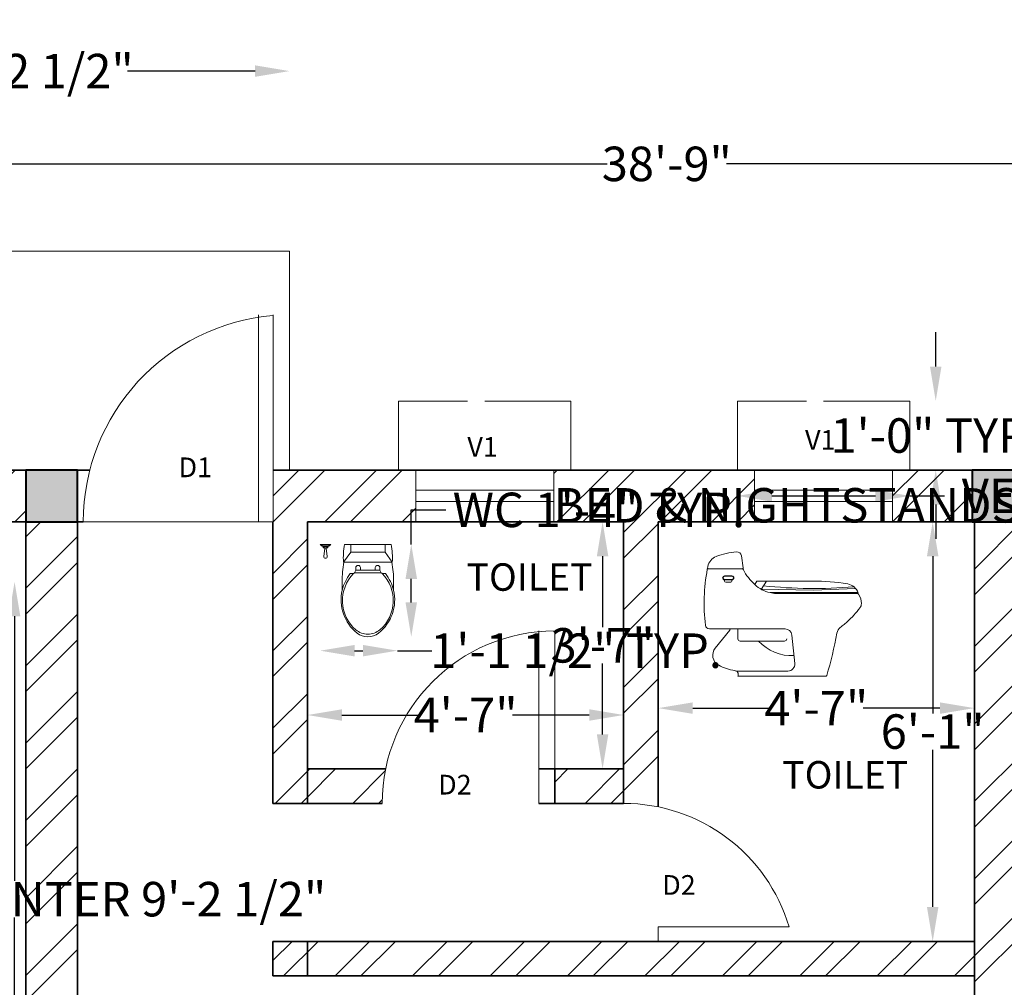
# Model space of a CAD drawing. Units: inches. Extents: x 3614 to 4242, y 2406 to 3033.
# Tile 8 of 10: x 3808 to 3980, y 2864 to 3033. Entities that reach past the tile are written whole.
import ezdxf

# ---------------------------------------------------------------- set-up
doc = ezdxf.new("R2010")
doc.units = ezdxf.units.IN
doc.linetypes.add('ACAD_ISO02W100', pattern=[15, 12, -3])
for name, color, linetype, lineweight in [('A-ANNO-DIMS', 2, 'Continuous', 18), ('A-ANNO-TEXT', 7, 'Continuous', 18), ('A-AREA-IDEN', 7, 'Continuous', 25), ('A-COLS', 7, 'Continuous', 40), ('A-COLS-PATT', 252, 'Continuous', 18), ('A-DOOR', 3, 'Continuous', 18), ('A-FLOR-FIXT', 9, 'Continuous', 18), ('A-FLOR-STRS', 7, 'Continuous', 18), ('A-GLAZ', 4, 'Continuous', 18), ('A-GLAZ-OVHD', 8, 'ACAD_ISO02W100', 13), ('A-WALL', 7, 'Continuous', 35), ('A-WALL-PATT', 252, 'Continuous', 13), ('WC-Detail_dwgmodels.com', 240, 'Continuous', 13), ('WC-Outline_dwgmodels.com', 250, 'Continuous', 18)]:
    doc.layers.add(name, color=color, linetype=linetype, lineweight=lineweight)
doc.styles.get("Standard").update_dxf_attribs({"font": 'arial.ttf'})
doc.dimstyles.get("Standard").update_dxf_attribs({"dimtxt": 6, "dimasz": 6, "dimexe": 0.18, "dimexo": 0.0625, "dimgap": 0.09, "dimtad": 0, "dimtih": 1, "dimtoh": 1, "dimdec": 4, "dimzin": 0, "dimdsep": 46, "dimlunit": 4, "dimtxsty": 'Standard', "dimcen": 0.09, "dimse1": 1, "dimse2": 1, "dimadec": 0, "dimazin": 0, "dimtfac": 1, "dimtdec": 4, "dimtofl": 0, "dimtmove": 0, "dimatfit": 3, "dimfxl": 1, "dimtolj": 1, "dimtzin": 0, "dimarcsym": 0})

# ---------------------------------------------------------------- blocks, each defined once
blk = doc.blocks.new('*D10')
at = {"layer": 'A-ANNO-DIMS', "color": 0, "lineweight": -2, "transparency": 16777216}
for p, q in [((3909.67, 2939.34), (3909.67, 2927)), ((3909.67, 2908.34), (3909.67, 2920.69))]:
    blk.add_line(p, q, dxfattribs=at)
at = {"layer": 'A-ANNO-DIMS', "color": 0, "transparency": 16777216}
for points in [[(3908.67, 2939.34), (3910.67, 2939.34), (3909.67, 2945.34)], [(3908.67, 2908.34), (3910.67, 2908.34), (3909.67, 2902.34)]]:
    blk.add_solid(points, dxfattribs=at)
at = {"layer": 'Defpoints', "color": 0, "transparency": 16777216}
for p in [(3909.37, 2945.34), (3909.37, 2902.34), (3909.67, 2902.34)]:
    blk.add_point(p, dxfattribs=at)
at = {"layer": 'A-ANNO-DIMS', "color": 0, "transparency": 16777216, "insert": (3909.67, 2923.84), "char_height": 6, "attachment_point": 5}
blk.add_mtext('\\A1;3\'-7"', dxfattribs=at)
blk = doc.blocks.new('*D11')
at = {"layer": 'A-ANNO-DIMS', "color": 0, "lineweight": -2, "transparency": 16777216}
for p, q in [((3864.34, 2911.72), (3877.65, 2911.72)), ((3907.34, 2911.72), (3894.02, 2911.72))]:
    blk.add_line(p, q, dxfattribs=at)
at = {"layer": 'A-ANNO-DIMS', "color": 0, "transparency": 16777216}
for points in [[(3864.34, 2912.72), (3864.34, 2910.72), (3858.34, 2911.72)], [(3907.34, 2912.72), (3907.34, 2910.72), (3913.34, 2911.72)]]:
    blk.add_solid(points, dxfattribs=at)
at = {"layer": 'Defpoints', "color": 0, "transparency": 16777216}
for p in [(3858.34, 2917.87), (3913.34, 2917.87), (3913.34, 2911.72)]:
    blk.add_point(p, dxfattribs=at)
at = {"layer": 'A-ANNO-DIMS', "color": 0, "transparency": 16777216, "insert": (3885.84, 2911.72), "char_height": 6, "attachment_point": 5}
blk.add_mtext('\\A1;4\'-7"', dxfattribs=at)
blk = doc.blocks.new('*D12')
at = {"layer": 'A-ANNO-DIMS', "color": 0, "lineweight": -2, "transparency": 16777216}
for p, q in [((3967.09, 2939.34), (3967.09, 2911.99)), ((3967.09, 2878.34), (3967.09, 2905.69))]:
    blk.add_line(p, q, dxfattribs=at)
at = {"layer": 'A-ANNO-DIMS', "color": 0, "transparency": 16777216}
for points in [[(3966.09, 2939.34), (3968.09, 2939.34), (3967.09, 2945.34)], [(3966.09, 2878.34), (3968.09, 2878.34), (3967.09, 2872.34)]]:
    blk.add_solid(points, dxfattribs=at)
at = {"layer": 'Defpoints', "color": 0, "transparency": 16777216}
for p in [(3966.94, 2945.34), (3966.94, 2872.34), (3967.09, 2872.34)]:
    blk.add_point(p, dxfattribs=at)
at = {"layer": 'A-ANNO-DIMS', "color": 0, "transparency": 16777216, "insert": (3967.09, 2908.84), "char_height": 6, "attachment_point": 5}
blk.add_mtext('\\A1;6\'-1"', dxfattribs=at)
blk = doc.blocks.new('*D13')
at = {"layer": 'A-ANNO-DIMS', "color": 0, "lineweight": -2, "transparency": 16777216}
for p, q in [((3925.34, 2912.92), (3938.65, 2912.92)), ((3968.34, 2912.92), (3955.02, 2912.92))]:
    blk.add_line(p, q, dxfattribs=at)
at = {"layer": 'A-ANNO-DIMS', "color": 0, "transparency": 16777216}
for points in [[(3925.34, 2913.92), (3925.34, 2911.92), (3919.34, 2912.92)], [(3968.34, 2913.92), (3968.34, 2911.92), (3974.34, 2912.92)]]:
    blk.add_solid(points, dxfattribs=at)
at = {"layer": 'Defpoints', "color": 0, "transparency": 16777216}
for p in [(3919.34, 2912.92), (3974.34, 2912.92), (3974.34, 2912.92)]:
    blk.add_point(p, dxfattribs=at)
at = {"layer": 'A-ANNO-DIMS', "color": 0, "transparency": 16777216, "insert": (3946.84, 2912.92), "char_height": 6, "attachment_point": 5}
blk.add_mtext('\\A1;4\'-7"', dxfattribs=at)
blk = doc.blocks.new('*D24')
at = {"layer": 'A-ANNO-DIMS', "color": 0, "lineweight": -2, "transparency": 16777216}
for p, q in [((3694.34, 3007.6), (3910.44, 3007.6)), ((4147.34, 3007.6), (3931.23, 3007.6))]:
    blk.add_line(p, q, dxfattribs=at)
at = {"layer": 'A-ANNO-DIMS', "color": 0, "transparency": 16777216}
for points in [[(3694.34, 3008.6), (3694.34, 3006.6), (3688.34, 3007.6)], [(4147.34, 3008.6), (4147.34, 3006.6), (4153.34, 3007.6)]]:
    blk.add_solid(points, dxfattribs=at)
at = {"layer": 'Defpoints', "color": 0, "transparency": 16777216}
for p in [(4153.34, 3007.6), (3688.34, 2954.34), (4153.34, 2954.34)]:
    blk.add_point(p, dxfattribs=at)
at = {"layer": 'A-ANNO-DIMS', "color": 0, "transparency": 16777216, "insert": (3920.84, 3007.6), "char_height": 6, "attachment_point": 5}
blk.add_mtext('\\A1;38\'-9"', dxfattribs=at)
blk = doc.blocks.new('VENT-V1-24IN')
for p, q in [((24, 9), (0, 9)), ((0, 9), (0, 0)), ((24, 0), (24, 9)), ((0, 5.5), (24, 5.5)), ((0, 3.5), (24, 3.5)), ((0, 0), (24, 0))]:
    blk.add_line(p, q)
blk = doc.blocks.new('SHADE-V1')
for p, q in [((0, 0), (0, 12)), ((0, 12), (27, 12)), ((27, 12), (30, 12)), ((30, 12), (30, 0)), ((3, 0), (0, 0))]:
    blk.add_line(p, q)
blk = doc.blocks.new('COLUMN-9X9')
blk.add_lwpolyline([(9, 9), (0, 9), (0, 0), (9, 0)], close=True)
blk = doc.blocks.new('DOOR-SWING-30IN')
for p, q in [((0, 30), (0, 0)), ((2.75, 30), (2.75, 0)), ((0, 0), (2.75, 0))]:
    blk.add_line(p, q)
blk.add_arc((0, 0), 30, 0, 90)
blk = doc.blocks.new('WC-PLAN')
for p, q in [((6.2, 11.58), (6.2, 12.03)), ((7.01, 12.03), (7.01, 11.58)), ((9.59, 12.03), (9.59, 11.58)), ((10.39, 11.58), (10.39, 12.03)), ((5.97, 11.16), (6.2, 11.58)), ((7.01, 11.58), (6.2, 11.58)), ((8.3, 11.58), (7.01, 11.58)), ((8.3, 11.58), (9.59, 11.58)), ((9.59, 11.58), (10.39, 11.58)), ((10.62, 11.16), (10.39, 11.58))]:
    blk.add_line(p, q)
for points in [[(1.85, 16.08), (0, 16.08)], [(1.73, 15.95), (0.11, 15.95)], [(1.35, 15.74), (0.5, 15.74)], [(0.5, 15.74), (0.5, 15.47), (0.8, 15.47)], [(0.72, 15.74), (0.72, 15.47)], [(0.8, 15.47), (1.07, 15.47)], [(1.07, 15.47), (1.34, 15.47), (1.35, 15.74)], [(1.15, 15.74), (1.15, 15.47)], [(4.05, 12.98), (5.32, 14.75), (5.32, 16.08)], [(12.37, 16.08), (4.22, 16.08)], [(12.54, 12.98), (11.28, 14.75), (11.28, 16.08)], [(5.32, 14.75), (8.3, 14.75)], [(11.28, 14.75), (8.3, 14.75)], [(4.13, 12.98), (8.3, 12.98)], [(12.47, 12.98), (8.3, 12.98)]]:
    blk.add_lwpolyline(points)
for points in [[(0.5, 15.74, -0.158381), (0, 16.08, 2.932383)], [(0.8, 15.45), (0.63, 13.98, 0.482607), (0.95, 13.67, -0.547905)], [(1.07, 15.45), (1.23, 13.98, -0.482607), (0.92, 13.67, 0.547905)], [(1.35, 15.74, 0.158381), (1.85, 16.08, -2.932383)], [(4.22, 16.08, 0.056711), (4.05, 12.98), (4.13, 12.98)], [(12.37, 16.08, -0.056711), (12.54, 12.98), (12.47, 12.98)], [(4.13, 12.98, 0.052121), (3.84, 9.61), (3.84, 8.13, 0.14456)], [(12.47, 12.98, -0.052121), (12.76, 9.61), (12.76, 8.13, -0.14456)], [(5.24, 11, 0.11024), (3.84, 8.13, 0.16845)], [(5.8, 11, 0.434217), (6.2, 1.23, 0.182634), (8.3, 0.47, 2.693815)], [(5.8, 11), (5.24, 11, 0.416606)], [(5.97, 11.16, 0.008985), (5.8, 11, 0.182634)], [(8.3, 11.16), (5.97, 11.16, 0.008985)], [(8.3, 11.16), (10.62, 11.16, -0.444938)], [(10.79, 11, -0.434217), (10.39, 1.23, -0.182634), (8.3, 0.47, -2.693815)], [(10.62, 11.16, -0.008985), (10.79, 11, -0.182634)], [(10.79, 11), (11.35, 11, -0.416606)], [(11.35, 11, -0.11024), (12.76, 8.13, -0.16845)], [(3.84, 8.13, 0.292914), (6.42, 0.65, 0.16845), (8.3, 0, 2.883082)], [(12.76, 8.13, -0.292914), (10.17, 0.65, -0.16845), (8.3, 0, -2.883082)]]:
    blk.add_lwpolyline(points, format="xyb")
for centre in [(6.6, 12.03), (9.99, 12.03)]:
    blk.add_arc(centre, 0.403, 0, 180)
blk = doc.blocks.new('*D51')
at = {"layer": 'A-ANNO-DIMS', "color": 0, "lineweight": -2, "transparency": 16777216}
for p, q in [((3939.12, 2949.84), (3957.12, 2949.84)), ((3963.12, 2949.84), (3969.12, 2949.84))]:
    blk.add_line(p, q, dxfattribs=at)
at = {"layer": 'A-ANNO-DIMS', "color": 0, "transparency": 16777216}
for points in [[(3939.12, 2950.84), (3939.12, 2948.84), (3933.12, 2949.84)], [(3957.12, 2950.84), (3957.12, 2948.84), (3963.12, 2949.84)]]:
    blk.add_solid(points, dxfattribs=at)
at = {"layer": 'Defpoints', "color": 0, "transparency": 16777216}
for p in [(3933.12, 2954.34), (3963.12, 2954.34), (3963.12, 2949.84)]:
    blk.add_point(p, dxfattribs=at)
at = {"layer": 'A-ANNO-DIMS', "color": 0, "transparency": 16777216, "insert": (4015.6, 2949.84), "char_height": 6, "attachment_point": 5}
blk.add_mtext('\\A1;VENT SHADE 2\'-6" TYP.', dxfattribs=at)
blk = doc.blocks.new('*D52')
at = {"layer": 'A-ANNO-DIMS', "color": 0, "lineweight": -2, "transparency": 16777216}
for p, q in [((3967.62, 2972.34), (3967.62, 2978.34)), ((3967.62, 2948.34), (3967.62, 2942.34))]:
    blk.add_line(p, q, dxfattribs=at)
at = {"layer": 'A-ANNO-DIMS', "color": 0, "transparency": 16777216}
for points in [[(3966.62, 2972.34), (3968.62, 2972.34), (3967.62, 2966.34)], [(3966.62, 2948.34), (3968.62, 2948.34), (3967.62, 2954.34)]]:
    blk.add_solid(points, dxfattribs=at)
at = {"layer": 'Defpoints', "color": 0, "transparency": 16777216}
for p in [(3963.12, 2966.34), (3967.62, 2966.34), (3963.12, 2954.34)]:
    blk.add_point(p, dxfattribs=at)
at = {"layer": 'A-ANNO-DIMS', "color": 0, "transparency": 16777216, "insert": (3967.62, 2960.34), "char_height": 6, "attachment_point": 5}
blk.add_mtext('\\A1;1\'-0" TYP.', dxfattribs=at)
blk = doc.blocks.new('*D55')
at = {"layer": 'A-ANNO-DIMS', "color": 0, "lineweight": -2, "transparency": 16777216}
for p, q in [((3876.39, 2941.41), (3876.39, 2947.41)), ((3876.39, 2947.41), (3882.39, 2947.41)), ((3876.39, 2931.32), (3876.39, 2935.41))]:
    blk.add_line(p, q, dxfattribs=at)
at = {"layer": 'A-ANNO-DIMS', "color": 0, "transparency": 16777216}
for points in [[(3875.39, 2935.41), (3877.39, 2935.41), (3876.39, 2941.41)], [(3875.39, 2931.32), (3877.39, 2931.32), (3876.39, 2925.32)]]:
    blk.add_solid(points, dxfattribs=at)
at = {"layer": 'Defpoints', "color": 0, "transparency": 16777216}
for p in [(3873.97, 2941.41), (3876.39, 2941.41), (3873.97, 2925.32)]:
    blk.add_point(p, dxfattribs=at)
at = {"layer": 'A-ANNO-DIMS', "color": 0, "transparency": 16777216, "insert": (3909.03, 2947.41), "char_height": 6, "attachment_point": 5}
blk.add_mtext('\\A1;WC 1\'-4" TYP.', dxfattribs=at)
blk = doc.blocks.new('*D56')
at = {"layer": 'A-ANNO-DIMS', "color": 0, "lineweight": -2, "transparency": 16777216}
for p, q in [((3866.54, 2922.91), (3867.97, 2922.91)), ((3873.97, 2922.91), (3879.97, 2922.91))]:
    blk.add_line(p, q, dxfattribs=at)
at = {"layer": 'A-ANNO-DIMS', "color": 0, "transparency": 16777216}
for points in [[(3866.54, 2923.91), (3866.54, 2921.91), (3860.54, 2922.91)], [(3867.97, 2923.91), (3867.97, 2921.91), (3873.97, 2922.91)]]:
    blk.add_solid(points, dxfattribs=at)
at = {"layer": 'Defpoints', "color": 0, "transparency": 16777216}
for p in [(3860.54, 2925.32), (3873.97, 2925.32), (3873.97, 2922.91)]:
    blk.add_point(p, dxfattribs=at)
at = {"layer": 'A-ANNO-DIMS', "color": 0, "transparency": 16777216, "insert": (3905.06, 2922.91), "char_height": 6, "attachment_point": 5}
blk.add_mtext('\\A1;1\'-1 1/2" TYP.', dxfattribs=at)
blk = doc.blocks.new('*D57')
at = {"layer": 'A-ANNO-DIMS', "color": 0, "lineweight": -2, "transparency": 16777216}
for p, q in [((4030.09, 2948.2), (4024.09, 2948.2)), ((4099.2, 2948.2), (4036.09, 2948.2))]:
    blk.add_line(p, q, dxfattribs=at)
at = {"layer": 'A-ANNO-DIMS', "color": 0, "transparency": 16777216}
for points in [[(4036.09, 2949.2), (4036.09, 2947.2), (4030.09, 2948.2)], [(4099.2, 2949.2), (4099.2, 2947.2), (4105.2, 2948.2)]]:
    blk.add_solid(points, dxfattribs=at)
at = {"layer": 'Defpoints', "color": 0, "transparency": 16777216}
for p in [(4030.09, 2948.2), (4030.09, 2936.94), (4105.2, 2936.94)]:
    blk.add_point(p, dxfattribs=at)
at = {"layer": 'A-ANNO-DIMS', "color": 0, "transparency": 16777216, "insert": (3960.9, 2948.2), "char_height": 6, "attachment_point": 5}
blk.add_mtext('\\A1;BED & NIGHTSTANDS 6\'-3" TYP.', dxfattribs=at)
blk = doc.blocks.new('*D63')
at = {"layer": 'A-ANNO-DIMS', "color": 0, "lineweight": -2, "transparency": 16777216}
for p, q in [((3807.39, 2928.9), (3807.39, 2882.88)), ((3807.39, 2830.46), (3807.39, 2876.49))]:
    blk.add_line(p, q, dxfattribs=at)
at = {"layer": 'A-ANNO-DIMS', "color": 0, "transparency": 16777216}
for points in [[(3806.39, 2928.9), (3808.39, 2928.9), (3807.39, 2934.9)], [(3806.39, 2830.46), (3808.39, 2830.46), (3807.39, 2824.46)]]:
    blk.add_solid(points, dxfattribs=at)
at = {"layer": 'Defpoints', "color": 0, "transparency": 16777216}
for p in [(3790.82, 2934.9), (3807.39, 2934.9), (3790.82, 2824.46)]:
    blk.add_point(p, dxfattribs=at)
at = {"layer": 'A-ANNO-DIMS', "color": 0, "transparency": 16777216, "insert": (3807.39, 2879.68), "char_height": 6, "attachment_point": 5}
blk.add_mtext('\\A1;KITCHEN COUNTER 9\'-2 1/2"', dxfattribs=at)
blk = doc.blocks.new('*D71')
at = {"layer": 'A-ANNO-DIMS', "color": 0, "lineweight": -2, "transparency": 16777216}
for p, q in [((3774.81, 3023.74), (3796.98, 3023.74)), ((3849.22, 3023.74), (3827.04, 3023.74))]:
    blk.add_line(p, q, dxfattribs=at)
at = {"layer": 'A-ANNO-DIMS', "color": 0, "transparency": 16777216}
for points in [[(3774.81, 3024.74), (3774.81, 3022.74), (3768.81, 3023.74)], [(3849.22, 3024.74), (3849.22, 3022.74), (3855.22, 3023.74)]]:
    blk.add_solid(points, dxfattribs=at)
at = {"layer": 'Defpoints', "color": 0, "transparency": 16777216}
for p in [(3855.22, 3023.74), (3768.81, 2992.44), (3855.22, 2992.44)]:
    blk.add_point(p, dxfattribs=at)
at = {"layer": 'A-ANNO-DIMS', "color": 0, "transparency": 16777216, "insert": (3812.01, 3023.74), "char_height": 6, "attachment_point": 5}
blk.add_mtext('\\A1;7\'-2 1/2"', dxfattribs=at)

msp = doc.modelspace()

# ---------------------------------------------------------------- hatches: boundary and pattern name
at = {"layer": 'A-COLS-PATT'}
h = msp.add_hatch(color=256, dxfattribs=at)
h.dxf.hatch_style = 1
h.paths.add_polyline_path([(3697.336, 2954.34049), (3688.336, 2954.34049), (3688.336, 2945.34049), (3697.336, 2945.34049)])
h.paths.add_polyline_path([(3818.336, 2954.34049), (3809.336, 2954.34049), (3809.336, 2945.34049), (3818.336, 2945.34049)])
h.paths.add_polyline_path([(3818.336, 2787.28572), (3809.336, 2787.28572), (3809.336, 2778.34049), (3818.336, 2778.34049)])
h.paths.add_polyline_path([(3697.336, 2742.34049), (3688.336, 2742.34049), (3688.336, 2733.34049), (3697.336, 2733.34049)])
h.paths.add_polyline_path([(3697.336, 2583.37355), (3688.336, 2583.37355), (3688.336, 2574.37355), (3697.336, 2574.37355)])
h.paths.add_polyline_path([(3899.336, 2583.34049), (3890.336, 2583.34049), (3890.336, 2574.34049), (3899.336, 2574.34049)])
h.paths.add_polyline_path([(3983.336, 2583.34049), (3974.336, 2583.34049), (3974.336, 2574.34049), (3983.336, 2574.34049)])
h.paths.add_polyline_path([(4153.336, 2583.34049), (4144.336, 2583.34049), (4144.336, 2574.34049), (4153.336, 2574.34049)])
h.paths.add_polyline_path([(4153.336, 2742.34049), (4144.336, 2742.34049), (4144.336, 2733.34049), (4153.336, 2733.34049)])
h.paths.add_polyline_path([(4153.336, 2795.34049), (4144.336, 2795.34049), (4144.336, 2786.34049), (4153.336, 2786.34049)])
h.paths.add_polyline_path([(3983.336, 2795.31105), (3974.336, 2795.31105), (3974.336, 2786.34049), (3983.336, 2786.34049)])
h.paths.add_polyline_path([(4153.336, 2954.34049), (4144.36882, 2954.34049), (4144.36882, 2945.34049), (4153.336, 2945.34049)])
h.paths.add_polyline_path([(3982.96188, 2954.34049), (3973.96188, 2954.34049), (3973.96188, 2945.34049), (3982.96188, 2945.34049)])
at = {"layer": 'A-WALL-PATT'}
h = msp.add_hatch(dxfattribs=at)
h.set_pattern_fill('ANSI32', color=256)
h.paths.add_polyline_path([(4041.01458, 2954.34049), (3982.96188, 2954.34049), (3982.96188, 2945.34049), (3983.336, 2945.34049), (4041.01458, 2945.34049)])
h.paths.add_polyline_path([(3973.96188, 2954.34049), (3960.11861, 2954.34049), (3960.11861, 2945.34049), (3973.96188, 2945.34049)])
h.paths.add_polyline_path([(3936.11861, 2954.34049), (3901.17016, 2954.34049), (3901.17016, 2945.34049), (3913.336, 2945.34049), (3913.336, 2896.34049, -0.050382044), (3919.336, 2895.73437), (3919.336, 2945.34049), (3936.11861, 2945.34049)])
h.paths.add_polyline_path([(3983.336, 2945.34049), (3982.96188, 2945.34049), (3974.336, 2945.34049), (3974.336, 2873.34049), (3974.336, 2795.31105), (3983.336, 2795.31105), (3983.336, 2867.34049)])
h.paths.add_polyline_path([(3974.336, 2872.34049), (3919.336, 2872.34049), (3858.336, 2872.34049), (3858.336, 2866.34049), (3919.336, 2866.34049), (3974.336, 2866.34049)])
h.paths.add_polyline_path([(3877.17016, 2954.34049), (3852.34021, 2954.34049), (3852.34021, 2945.34049), (3852.336, 2896.34049), (3858.336, 2896.34049), (3858.336, 2945.34049), (3877.17016, 2945.34049)])
h.paths.add_polyline_path([(3871.94212, 2902.34049), (3858.336, 2902.34049), (3858.336, 2896.34049), (3871.336, 2896.34049, -0.050382044)], flags=0)
h.paths.add_polyline_path([(3913.336, 2902.34049), (3901.336, 2902.34049), (3901.336, 2896.34049), (3913.336, 2896.34049)], flags=17)
h.paths.add_polyline_path([(3858.336, 2872.34049), (3852.336, 2872.34049), (3852.336, 2866.34049), (3858.336, 2866.34049)])
h.paths.add_polyline_path([(3809.336, 2954.34049), (3764.4617, 2954.34049), (3764.4617, 2945.34049), (3809.336, 2945.34049)])
h.paths.add_polyline_path([(3716.4617, 2954.34049), (3697.336, 2954.34049), (3697.336, 2945.34049), (3716.4617, 2945.34049)])
h.paths.add_polyline_path([(3697.336, 2945.34049), (3688.336, 2945.34049), (3688.336, 2894.73438), (3697.336, 2894.73438)])
h = msp.add_hatch(dxfattribs=at)
h.set_pattern_fill('ANSI32', color=256)
h.paths.add_polyline_path([(4153.336, 2945.34049), (4144.336, 2945.34049), (4144.336, 2902.95478), (4153.336, 2902.95478)])
h.paths.add_polyline_path([(4144.36882, 2954.34049), (4089.01458, 2954.34049), (4089.01458, 2945.34049), (4144.36882, 2945.34049)])
h.paths.add_polyline_path([(3818.336, 2945.34049), (3809.336, 2945.34049), (3809.336, 2787.28572), (3818.336, 2787.28572)])
h.paths.add_polyline_path([(3697.336, 2846.73438), (3688.336, 2846.73438), (3688.336, 2742.34049), (3697.336, 2742.34049)])
h.paths.add_polyline_path([(3854.336, 2742.34049), (3853.36389, 2742.34049), (3818.336, 2742.34049), (3809.336, 2742.34049), (3697.336, 2742.34049), (3697.336, 2733.34049), (3809.336, 2733.34049), (3854.336, 2733.34049)])
h.paths.add_polyline_path([(3697.336, 2733.34049), (3688.336, 2733.34049), (3688.336, 2690.05693), (3697.336, 2690.05693)])
h.paths.add_polyline_path([(3697.336, 2642.05693), (3688.336, 2642.05693), (3688.336, 2583.37355), (3697.336, 2583.37355)])
h.paths.add_polyline_path([(3726.39802, 2583.34049), (3697.336, 2583.34049), (3697.336, 2574.34049), (3726.39802, 2574.34049)])
h.paths.add_polyline_path([(3842.336, 2583.34049), (3818.336, 2583.34049), (3809.336, 2583.34049), (3774.39802, 2583.34049), (3774.39802, 2574.34049), (3809.336, 2574.34049), (3842.336, 2574.34049)])
h.paths.add_polyline_path([(3890.336, 2583.34049), (3878.336, 2583.34049), (3878.336, 2574.34049), (3890.336, 2574.34049)])
h = msp.add_hatch(dxfattribs=at)
h.set_pattern_fill('ANSI32', color=256)
h.paths.add_polyline_path([(3871.94212, 2902.34049), (3858.336, 2902.34049), (3858.336, 2896.34049), (3871.336, 2896.34049, -0.050382044)])

# ---------------------------------------------------------------- linework, layer by layer
at = {"layer": 'A-DOOR'}
for p, q in [((3849.84021, 2981.34049), (3849.84021, 2945.34049)), ((3852.34021, 2981.34049), (3852.34021, 2945.34049)), ((3819.34021, 2945.34049), (3852.336, 2945.34049)), ((3852.34021, 2945.34049), (3852.336, 2945.34049)), ((3919.336, 2874.84049), (3942.10664, 2874.84049)), ((3919.336, 2872.34049), (3919.336, 2874.84049))]:
    msp.add_line(p, q, dxfattribs=at)
for centre, radius, start, end in [((3855.34021, 2945.34049), 36, 94.7801918, 180), ((3913.336, 2866.34049), 30, 16.4592496, 90)]:
    msp.add_arc(centre, radius, start, end, dxfattribs=at)
at = {"layer": 'A-FLOR-STRS'}
for p, q in [((3768.80751, 2992.43626), (3855.21729, 2992.43626)), ((3855.21729, 2992.43626), (3855.21729, 2954.34049))]:
    msp.add_line(p, q, dxfattribs=at)
at = {"layer": 'A-WALL'}
for p, q in [((3688.336, 2954.34049), (3820.48336, 2954.34049)), ((3852.34021, 2954.34049), (4153.336, 2954.34049)), ((3697.336, 2945.34049), (3809.336, 2945.34049)), ((3809.336, 2945.34049), (3809.336, 2778.34049)), ((3818.336, 2945.34049), (3818.336, 2778.34049)), ((3818.336, 2945.34049), (3819.34021, 2945.34049)), ((3852.336, 2945.34049), (3852.336, 2896.34049)), ((3858.336, 2945.34049), (3858.336, 2896.34049)), ((3858.336, 2945.34049), (3913.336, 2945.34049)), ((3913.336, 2945.34049), (3913.336, 2896.34049)), ((3919.336, 2945.34049), (3919.336, 2895.73437)), ((3919.336, 2945.34049), (3974.336, 2945.34049)), ((3974.336, 2945.34049), (3974.336, 2873.34049)), ((3858.336, 2902.34049), (3871.94212, 2902.34049)), ((3898.586, 2902.34049), (3913.336, 2902.34049)), ((3913.336, 2902.34049), (3901.336, 2902.34049)), ((3901.336, 2902.34049), (3901.336, 2896.34049)), ((3858.336, 2896.34049), (3852.336, 2896.34049)), ((3858.336, 2896.34049), (3871.336, 2896.34049)), ((3898.586, 2896.34049), (3913.336, 2896.34049)), ((3901.336, 2896.34049), (3913.336, 2896.34049)), ((3858.336, 2872.34049), (3852.336, 2872.34049)), ((3852.336, 2872.34049), (3852.336, 2866.34049)), ((3919.336, 2872.34049), (3858.336, 2872.34049)), ((3858.336, 2872.34049), (3858.336, 2866.34049)), ((3919.336, 2872.34049), (3974.336, 2872.34049)), ((3974.336, 2873.34049), (3974.336, 2786.34049)), ((3919.336, 2866.34049), (3852.336, 2866.34049)), ((3943.336, 2866.34049), (3913.336, 2866.34049)), ((3919.336, 2866.34049), (3974.336, 2866.34049))]:
    msp.add_line(p, q, dxfattribs=at)
at = {"layer": 'WC-Detail_dwgmodels.com'}
for p, q in [((3928.04484, 2937.16827), (3933.87181, 2937.16827)), ((3930.89392, 2935.85109), (3932.16345, 2935.85109)), ((3930.89392, 2935.30698), (3932.16345, 2935.30698)), ((3930.89392, 2935.03099), (3930.89392, 2935.22813)), ((3931.09106, 2934.83386), (3931.96631, 2934.83386)), ((3932.16345, 2935.03099), (3932.16345, 2935.22813)), ((3937.2804, 2933.58178), (3938.19389, 2934.9953)), ((3933.19505, 2926.70086), (3933.19505, 2924.97491)), ((3933.58932, 2924.58064), (3941.30413, 2924.58064)), ((3933.21119, 2918.50008), (3933.25686, 2918.59143))]:
    msp.add_line(p, q, dxfattribs=at)
msp.add_lwpolyline([(3953.36637, 2934.03867, -0.050023446), (3937.683, 2934.20476, 1.562232991)], format="xyb", dxfattribs=at)
msp.add_lwpolyline([(3937.3046, 2933.61923), (3946.27352, 2933.42535), (3953.70735, 2933.70708)], dxfattribs=at)
for centre, radius, start, end in [((3930.89392, 2935.57903), 0.27205, 90, 270), ((3932.16345, 2935.57903), 0.27205, 270, 90), ((3931.09106, 2935.03099), 0.19713, 180, 270), ((3931.96631, 2935.03099), 0.19713, 270, 0), ((3933.58932, 2924.97491), 0.39427, 180, 270), ((3942.56603, 2929.82404), 7.78786, 222.3205859, 272.8267189), ((3941.30413, 2924.97491), 0.39427, 270, 0)]:
    msp.add_arc(centre, radius, start, end, dxfattribs=at)
at = {"layer": 'WC-Outline_dwgmodels.com'}
for p, q in [((3934.12467, 2937.30366), (3933.81392, 2939.4292)), ((3927.99881, 2937.16827), (3928.04484, 2937.16827)), ((3930.89392, 2935.92994), (3932.16345, 2935.92994)), ((3933.87181, 2937.16827), (3934.00763, 2937.16827)), ((3930.89392, 2935.22813), (3932.16345, 2935.22813)), ((3952.2104, 2927.94716), (3951.67146, 2927.46972)), ((3928.25729, 2926.70086), (3931.81277, 2926.70086)), ((3929.26226, 2923.37043), (3931.81277, 2926.50797)), ((3931.81277, 2926.70086), (3941.40927, 2926.70086)), ((3942.58604, 2925.63733), (3943.08957, 2920.66956)), ((3932.86275, 2919.36747), (3941.9128, 2919.36747)), ((3933.21119, 2918.50008), (3948.56595, 2918.50008))]:
    msp.add_line(p, q, dxfattribs=at)
msp.add_lwpolyline([(3936.16192, 2934.39634), (3936.48382, 2934.9953), (3946.18973, 2934.9953, -0.050027594), (3952.30455, 2934.51876, -0.265083568), (3954.1172, 2933.00436), (3951.83786, 2933.00436), (3938.79533, 2933.00436, 0.044731127), (3939.80089, 2932.8713), (3953.92857, 2932.8713)], format="xyb", dxfattribs=at)
for centre, radius, start, end in [((3930.29891, 2937.0941), 2.36561, 112.0681517, 168.2796563), ((3933.71215, 2928.67488), 11.4504, 93.6485285, 112.0681517), ((3933.03367, 2939.31513), 0.78854, 8.3176492, 93.6485285), ((3958.86645, 2931.16746), 31.54145, 168.2796563, 168.7709525), ((3959.24732, 2931.1316), 31.92231, 169.2751135, 186.8478168), ((3927.99881, 2937.04999), 0.11828, 90, 169.2103766), ((3928.04484, 2937.28655), 0.11828, 168.7709525, 270), ((3930.89392, 2935.57903), 0.35091, 90, 270), ((3932.16345, 2935.57903), 0.35091, 270, 90), ((3933.87181, 2936.85285), 0.31541, 26.8060073, 90), ((3934.00763, 2937.28655), 0.11828, 270, 8.3176492), ((3941.89512, 2940.90677), 8.6739, 206.8060073, 228.3973777), ((3940.04028, 2938.54662), 5.68037, 226.5808179, 226.9397607), ((3940.04028, 2938.54662), 5.68037, 226.9397607, 257.3398133), ((3953.92857, 2932.55588), 0.31541, 33.9938204, 90), ((3951.84775, 2931.12722), 2.83956, 359.3578247, 34.4197551), ((3953.50441, 2931.10873), 1.1828, 323.6662198, 359.3538915), ((3941.75269, 2939.7519), 15.77072, 311.5374256, 323.6662198), ((3928.25729, 2927.41054), 0.70968, 186.8890678, 270), ((3939.53336, 2941.94347), 18.88976, 307.4560919, 309.9841419), ((3931.72099, 2926.58258), 0.11828, 320.8922932, 90), ((3941.40927, 2925.51806), 1.1828, 5.787731, 90), ((3872.90791, 2940.41549), 78.85362, 343.9282752, 349.455321), ((3951.98033, 2925.6965), 1.57707, 127.4560919, 169.455321), ((3930.79194, 2922.12695), 1.97134, 140.8922932, 242.3685163), ((3934.27713, 2928.8087), 9.50741, 242.435904, 260.2462822), ((3941.9128, 2920.55028), 1.1828, 270, 5.787731), ((3932.60145, 2918.76408), 0.67777, 345.2425322, 84.496457), ((3948.56595, 2918.61836), 0.11828, 270, 343.9282752)]:
    msp.add_arc(centre, radius, start, end, dxfattribs=at)

# ---------------------------------------------------------------- block references
at = {"layer": 'A-COLS'}
for p in [(3809.336, 2945.34), (3973.96188, 2945.34)]:
    msp.add_blockref('COLUMN-9X9', p, dxfattribs=at)
at = {"layer": 'A-DOOR', "extrusion": (0, 0, -1), "zscale": -1}
msp.add_blockref('DOOR-SWING-30IN', (-3901.33594, 2896.34), dxfattribs=at)
at = {"layer": 'A-FLOR-FIXT'}
msp.add_blockref('WC-PLAN', (3860.544, 2925.323), dxfattribs=at)
at = {"layer": 'A-GLAZ', "extrusion": (0, 0, -1), "zscale": -1}
msp.add_blockref('VENT-V1-24IN', (-3901.16977, 2945.34), dxfattribs=at)
at = {"layer": 'A-GLAZ'}
msp.add_blockref('VENT-V1-24IN', (3936.119, 2945.34), dxfattribs=at)
at = {"layer": 'A-GLAZ-OVHD'}
for p in [(3874.17055, 2954.34), (3933.119, 2954.34)]:
    msp.add_blockref('SHADE-V1', p, dxfattribs=at)

# ---------------------------------------------------------------- texts
at = {"layer": 'A-ANNO-TEXT', "char_height": 3.42604, "attachment_point": 1}
for s, insert in [('V1', (3886.14756, 2960.06529)), ('V1', (3944.89239, 2961.27851)), ('D1', (3835.9222, 2956.51915)), ('D2', (3881.07355, 2901.3167)), ('D2', (3920.0517, 2883.86492))]:
    msp.add_mtext_dynamic_manual_height_columns(s, width=192.8287007, gutter_width=17.1302, heights=[0], dxfattribs=dict(at, insert=insert))
at = {"layer": 'A-AREA-IDEN', "char_height": 4.777705, "attachment_point": 1}
for s, insert in [('TOILET ', (3886.00557, 2938.10953)), ('TOILET', (3940.91398, 2903.70602))]:
    msp.add_mtext_dynamic_manual_height_columns(s, width=66.2541682, gutter_width=12.5, heights=[0], dxfattribs=dict(at, insert=insert))

# ---------------------------------------------------------------- dimensions: what is measured, and where the dimension line sits
at = {"layer": 'A-ANNO-DIMS'}
for base, p1, p2, override, picture, middle in [((3855.21729, 3023.73626), (3768.80751, 2992.43626), (3855.21729, 2992.43626), {"dimdec": 1, "dimlfac": 1, "dimrnd": 0, "dimzin": 1, "dimdsep": 46, "dimlunit": 4, "dimfrac": 2}, '*D71', (3812.0124, 3023.73626)), ((4153.336, 3007.59551), (3688.336, 2954.34049), (4153.336, 2954.34049), {"dimclrd": 0, "dimclre": 0, "dimclrt": 0}, '*D24', (3920.836, 3007.59551)), ((3913.336, 2911.71735), (3858.336, 2917.87166), (3913.336, 2917.87166), {"dimclrd": 0, "dimclre": 0, "dimclrt": 0}, '*D11', (3885.836, 2911.71735)), ((3974.336, 2912.91819), (3919.336, 2912.91819), (3974.336, 2912.91819), {"dimclrd": 0, "dimclre": 0, "dimclrt": 0}, '*D13', (3946.836, 2912.91819))]:
    dim = msp.add_linear_dim(base=base, p1=p1, p2=p2, dimstyle='Standard', override=override, dxfattribs=at)
    dim.commit()
    dim.dimension.update_dxf_attribs({"geometry": picture, "text_midpoint": middle})
for base, p1, p2, angle, text, picture, middle in [((3967.61861, 2966.34049), (3963.11861, 2954.34049), (3963.11861, 2966.34049), 90, '<> TYP.', '*D52', (3967.61861, 2960.34049)), ((4030.09092, 2948.20225), (4105.2039, 2936.9353), (4030.09092, 2936.9353), 180, 'BED & NIGHTSTANDS <> TYP.', '*D57', (3960.90474, 2948.20225)), ((3876.38578, 2941.40502), (3873.9735, 2925.3232), (3873.9735, 2941.40502), 90, 'WC <> TYP.', '*D55', (3909.03171, 2947.40502)), ((3807.38582, 2934.90029), (3790.82041, 2824.46424), (3790.82041, 2934.90029), 90, 'KITCHEN COUNTER <>', '*D63', (3807.38582, 2879.68227))]:
    dim = msp.add_linear_dim(base=base, p1=p1, p2=p2, angle=angle, text=text, dimstyle='Standard', override={"dimdec": 1, "dimlfac": 1, "dimrnd": 0, "dimzin": 1, "dimdsep": 46, "dimlunit": 4, "dimfrac": 2}, dxfattribs=at)
    dim.commit()
    dim.dimension.update_dxf_attribs({"geometry": picture, "text_midpoint": middle})
for base, p1, p2, text, picture, middle in [((3963.11861, 2949.84049), (3933.11861, 2954.34049), (3963.11861, 2954.34049), 'VENT SHADE <> TYP.', '*D51', (4015.59606, 2949.84049)), ((3873.9735, 2922.91092), (3860.5439, 2925.3232), (3873.9735, 2925.3232), '<> TYP.', '*D56', (3905.05804, 2922.91092))]:
    dim = msp.add_linear_dim(base=base, p1=p1, p2=p2, text=text, dimstyle='Standard', override={"dimdec": 1, "dimlfac": 1, "dimrnd": 0, "dimzin": 1, "dimdsep": 46, "dimlunit": 4, "dimfrac": 2}, dxfattribs=at)
    dim.commit()
    dim.dimension.update_dxf_attribs({"geometry": picture, "text_midpoint": middle})
for base, p1, p2, picture, middle in [((3909.66622, 2902.34049), (3909.36504, 2945.34049), (3909.36504, 2902.34049), '*D10', (3909.66622, 2923.84049)), ((3967.09288, 2872.34049), (3966.94269, 2945.34049), (3966.94269, 2872.34049), '*D12', (3967.09288, 2908.84049))]:
    dim = msp.add_linear_dim(base=base, p1=p1, p2=p2, angle=90, dimstyle='Standard', override={"dimclrd": 0, "dimclre": 0, "dimclrt": 0}, dxfattribs=at)
    dim.commit()
    dim.dimension.update_dxf_attribs({"geometry": picture, "text_midpoint": middle})

doc.saveas('drawing.dxf')
